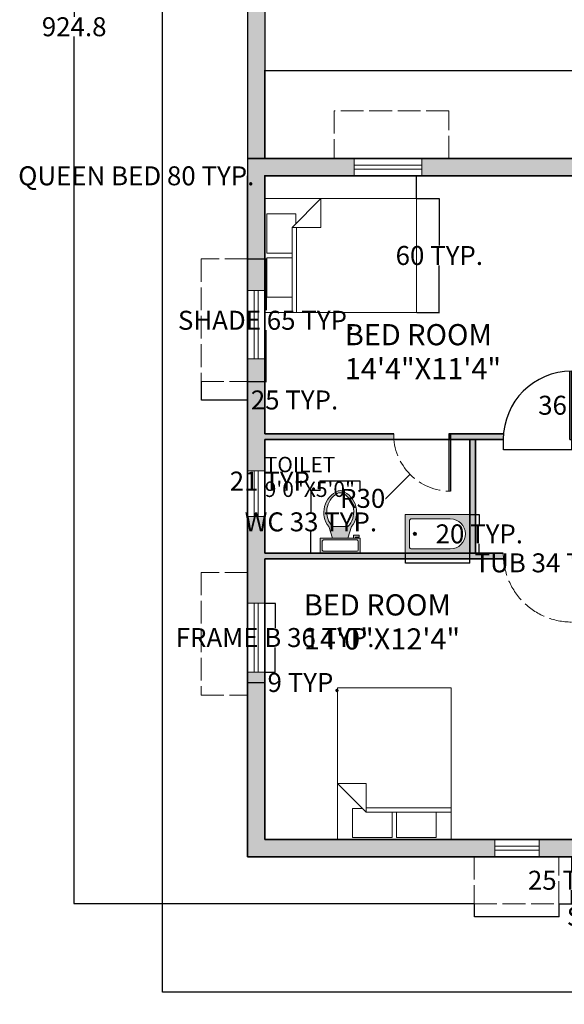
# Model space of a CAD drawing. Units: inches. Extents: x 215 to 969, y -612 to 418.
# Tile 1 of 8: x 215 to 502, y -612 to -93. Entities that reach past the tile are written whole.
import ezdxf

# ---------------------------------------------------------------- set-up
doc = ezdxf.new("R2010")
doc.units = ezdxf.units.IN
doc.header["$MEASUREMENT"] = 0
doc.linetypes.add('ACAD_ISO02W100', pattern=[15, 12, -3])
for name, color, linetype, lineweight in [('A-ANNO-DIMS', 2, 'Continuous', 18), ('A-AREA-IDEN', 7, 'Continuous', 18), ('A-DOOR', 3, 'Continuous', 25), ('A-DOOR-SWNG', 3, 'ACAD_ISO02W100', 13), ('A-FLOR-FIXT', 9, 'Continuous', 18), ('A-FLOR-OVHD', 8, 'ACAD_ISO02W100', 13), ('A-FLOR-SLAB', 7, 'Continuous', 25), ('A-FURN', 8, 'Continuous', 18), ('A-GLAZ', 4, 'Continuous', 18), ('A-WALL', 7, 'Continuous', 35)]:
    doc.layers.add(name, color=color, linetype=linetype, lineweight=lineweight)
doc.layers.add('A-WALL-PATT', color=252, linetype='Continuous', lineweight=13, true_color=0x939598)
doc.styles.get("Standard").update_dxf_attribs({"font": 'arial.ttf'})
doc.dimstyles.get("Standard").update_dxf_attribs({"dimtxt": 10, "dimasz": 0.18, "dimexe": 0.18, "dimexo": 0.0625, "dimgap": 0.09, "dimtad": 0, "dimtih": 1, "dimtoh": 1, "dimdec": 0, "dimzin": 0, "dimdsep": 46, "dimlunit": 3, "dimtxsty": 'Standard', "dimcen": 0.09, "dimadec": 0, "dimazin": 0, "dimtfac": 1, "dimtdec": 0, "dimtofl": 0, "dimtmove": 0, "dimatfit": 3, "dimfxl": 1, "dimtolj": 1, "dimtzin": 0, "dimarcsym": 0})

# ---------------------------------------------------------------- blocks, each defined once
blk = doc.blocks.new('Bed - Queen')
for p, q in [((0, -80.00003), (0, 0)), ((0, 0), (59.99999, 0)), ((59.99999, 0), (59.99999, -80.00003)), ((7.99999, -1.2), (28.79998, -1.2)), ((7.99999, -14.4), (7.99999, -1.2)), ((28.79998, -1.2), (28.79998, -14.4)), ((31.19999, -1.2), (51.99999, -1.2)), ((31.19999, -14.4), (31.19999, -1.2)), ((51.99999, -1.2), (51.99999, -16.4)), ((0, -14.4), (44.8, -14.4)), ((59.99999, -29.6), (44.8, -14.4)), ((44.8, -14.4), (44.8, -29.6)), ((44.8, -16.8), (0, -16.8)), ((51.99999, -16.4), (46.79936, -16.4)), ((44.8, -29.6), (59.99999, -29.6)), ((59.99999, -80.00003), (0, -80.00003))]:
    blk.add_line(p, q)
blk = doc.blocks.new('Bath Tub - 26 x 60 in.')
for p, q in [((8, -18), (10, -18)), ((9, -17), (9, -19))]:
    blk.add_line(p, q)
blk.add_lwpolyline([(0, -36), (0, 0), (60, 0), (60, -36)], close=True)
for points in [[(4, -30), (4, -6)], [(6, -4), (42, -4)], [(42, -32), (6, -32)]]:
    blk.add_lwpolyline(points)
for radius in [1.5, 1]:
    blk.add_circle((9, -18), radius)
for centre, radius, start, end in [((5.75, -5.75), 1.77, 81.8699, 188.1301), ((42, -18), 14, 270, 90), ((5.75, -30.25), 1.77, 171.8699, 278.1301)]:
    blk.add_arc(centre, radius, start, end)
blk = doc.blocks.new('Toilet - top')
for p, q in [((9.5, -6), (9.5, -2)), ((-10, -8.5), (-8, -8.5)), ((-10, -9.5), (-10, -8.5)), ((-7, -9.5), (-10, -9.5)), ((-8, -8.5), (-8, -8)), ((-7, -8), (-7, -9.5)), ((-4, -8), (-6, -14)), ((4, -8), (6, -14)), ((4, -14), (-4, -14))]:
    blk.add_line(p, q)
blk.add_lwpolyline([(10.5, -8), (10.5, 0), (-10.5, 0), (-10.5, -8)], close=True)
for points in [[(-9.5, -2), (-9.5, -6)], [(8.5, -1), (-8.5, -1)], [(-8.5, -7), (8.5, -7)]]:
    blk.add_lwpolyline(points)
for centre, radius, start, end in [((-8.62, -1.88), 0.884, 81.8699, 188.1301), ((8.62, -1.88), 0.884, 351.8699, 98.1301), ((-8.62, -6.12), 0.884, 171.8699, 278.1301), ((8.62, -6.12), 0.884, 261.8699, 8.1301), ((3.52, -21.58), 12.17, 141.4691, 247.9714), ((4.2, -21.82), 11.33, 136.3677, 238.9468), ((-3.52, -21.58), 12.17, 292.0284, 38.5307), ((-4.2, -21.82), 11.33, 301.053, 43.6321), ((0, -27.88), 4, 245.7318, 294.2682), ((0, -29), 4, 254.8605, 285.1395)]:
    blk.add_arc(centre, radius, start, end)
blk = doc.blocks.new('WINDOW-SHADE-60')
for p, q in [((60.48, 25.28), (0, 25.28)), ((0, 25.28), (0, 0)), ((60.48, 0), (60.48, 25.28))]:
    blk.add_line(p, q)
blk = doc.blocks.new('WINDOW-SHADE-65')
for p, q in [((24.53, 64.64), (0, 64.64)), ((0, 64.64), (0, 0)), ((0, 0), (24.53, 0))]:
    blk.add_line(p, q)
blk = doc.blocks.new('WINDOW-SHADE-45')
for p, q in [((0, 24.86), (0, 0)), ((44.63, 0), (44.63, 24.86)), ((0, 0), (44.63, 0))]:
    blk.add_line(p, q)
blk = doc.blocks.new('DOOR-SINGLE-36')
for p, q in [((35, 0), (35, 36)), ((36, 0), (36, 36)), ((35, 0), (36, 0))]:
    blk.add_line(p, q)
blk.add_arc((36, 0), 36, 90, 180)
blk = doc.blocks.new('WIN-24')
for p, q in [((0, 9), (0, 0)), ((0, 5.5), (23.37, 5.5)), ((23.37, 9), (23.37, 0)), ((0, 3.5), (23.37, 3.5))]:
    blk.add_line(p, q)
blk = doc.blocks.new('WIN-FRAME-24B')
for p, q in [((0, 23.99), (9, 23.99)), ((3.5, 23.99), (3.5, 0)), ((5.5, 23.99), (5.5, 0)), ((9, 0), (0, 0)), ((4.5, 0), (9, 0))]:
    blk.add_line(p, q)
blk = doc.blocks.new('WIN-FRAME-36A')
for p, q in [((0, 35.94), (9, 35.94)), ((3.5, 35.94), (3.5, 0)), ((5.5, 35.94), (5.5, 0)), ((9, 0), (0, 0)), ((4.5, 0), (9, 0))]:
    blk.add_line(p, q)
blk = doc.blocks.new('WIN-FRAME-36B')
for p, q in [((9, 36.42), (0, 36.42)), ((3.5, 36.42), (3.5, 0)), ((5.5, 36.42), (5.5, 0)), ((4.5, 0), (0, 0)), ((0, 0), (9, 0))]:
    blk.add_line(p, q)
blk = doc.blocks.new('*D23')
at = {"layer": 'A-ANNO-DIMS', "color": 0, "lineweight": -2, "transparency": 16777216}
for p, q in [((344.35, -175.5), (344.17, -175.5)), ((344.35, -187.44), (344.35, -175.32)), ((424.17, -175.5), (344.53, -175.5)), ((424.35, -187.44), (424.35, -175.32))]:
    blk.add_line(p, q, dxfattribs=at)
at = {"layer": 'A-ANNO-DIMS', "color": 0, "transparency": 16777216}
for points in [[(344.53, -175.47), (344.53, -175.53), (344.35, -175.5)], [(424.17, -175.47), (424.17, -175.53), (424.35, -175.5)]]:
    blk.add_solid(points, dxfattribs=at)
at = {"layer": 'Defpoints', "color": 0, "transparency": 16777216}
for p in [(344.35, -175.5), (344.35, -187.5), (424.35, -187.5)]:
    blk.add_point(p, dxfattribs=at)
at = {"layer": 'A-ANNO-DIMS', "color": 0, "transparency": 16777216, "insert": (276.67, -175.5), "char_height": 10, "attachment_point": 5}
blk.add_mtext('\\A1;QUEEN BED 80 TYP.', dxfattribs=at)
blk = doc.blocks.new('*D24')
at = {"layer": 'A-ANNO-DIMS', "color": 0, "lineweight": -2, "transparency": 16777216}
for p, q in [((424.42, -187.5), (436.53, -187.5)), ((436.35, -187.68), (436.35, -212.31)), ((436.35, -247.32), (436.35, -222.7)), ((424.42, -247.5), (436.53, -247.5))]:
    blk.add_line(p, q, dxfattribs=at)
at = {"layer": 'A-ANNO-DIMS', "color": 0, "transparency": 16777216}
for points in [[(436.32, -187.68), (436.38, -187.68), (436.35, -187.5)], [(436.32, -247.32), (436.38, -247.32), (436.35, -247.5)]]:
    blk.add_solid(points, dxfattribs=at)
at = {"layer": 'Defpoints', "color": 0, "transparency": 16777216}
for p in [(424.35, -187.5), (436.35, -187.5), (424.35, -247.5)]:
    blk.add_point(p, dxfattribs=at)
at = {"layer": 'A-ANNO-DIMS', "color": 0, "transparency": 16777216, "insert": (436.35, -217.5), "char_height": 10, "attachment_point": 5}
blk.add_mtext('\\A1;60 TYP.', dxfattribs=at)
blk = doc.blocks.new('*D25')
at = {"layer": 'A-ANNO-DIMS', "color": 0, "lineweight": -2, "transparency": 16777216}
for p, q in [((373.57, -341.41), (368.5, -341.41)), ((368.68, -341.59), (368.68, -352.67)), ((368.68, -374.27), (368.68, -363.19)), ((373.57, -374.45), (368.5, -374.45))]:
    blk.add_line(p, q, dxfattribs=at)
at = {"layer": 'A-ANNO-DIMS', "color": 0, "transparency": 16777216}
for points in [[(368.65, -341.59), (368.71, -341.59), (368.68, -341.41)], [(368.65, -374.27), (368.71, -374.27), (368.68, -374.45)]]:
    blk.add_solid(points, dxfattribs=at)
at = {"layer": 'Defpoints', "color": 0, "transparency": 16777216}
for p in [(373.64, -341.41), (368.68, -374.45), (373.64, -374.45)]:
    blk.add_point(p, dxfattribs=at)
at = {"layer": 'A-ANNO-DIMS', "color": 0, "transparency": 16777216, "insert": (368.68, -357.93), "char_height": 10, "attachment_point": 5}
blk.add_mtext('\\A1;WC 33 TYP.', dxfattribs=at)
blk = doc.blocks.new('*D26')
at = {"layer": 'A-ANNO-DIMS', "color": 0, "lineweight": -2, "transparency": 16777216}
for p, q in [((373.64, -336.45), (373.46, -336.45)), ((373.64, -341.34), (373.64, -336.27)), ((394.46, -336.45), (373.82, -336.45)), ((394.64, -341.34), (394.64, -336.27))]:
    blk.add_line(p, q, dxfattribs=at)
at = {"layer": 'A-ANNO-DIMS', "color": 0, "transparency": 16777216}
for points in [[(373.82, -336.42), (373.82, -336.48), (373.64, -336.45)], [(394.46, -336.42), (394.46, -336.48), (394.64, -336.45)]]:
    blk.add_solid(points, dxfattribs=at)
at = {"layer": 'Defpoints', "color": 0, "transparency": 16777216}
for p in [(373.64, -336.45), (373.64, -341.41), (394.64, -341.41)]:
    blk.add_point(p, dxfattribs=at)
at = {"layer": 'A-ANNO-DIMS', "color": 0, "transparency": 16777216, "insert": (348.94, -336.45), "char_height": 10, "attachment_point": 5}
blk.add_mtext('\\A1;21 TYP.', dxfattribs=at)
blk = doc.blocks.new('*D33')
at = {"layer": 'A-ANNO-DIMS', "color": 0, "lineweight": -2, "transparency": 16777216}
for p, q in [((418.41, -374.51), (418.41, -379.72)), ((452.34, -374.51), (452.34, -379.72)), ((418.59, -379.54), (452.16, -379.54)), ((452.34, -379.54), (452.52, -379.54))]:
    blk.add_line(p, q, dxfattribs=at)
at = {"layer": 'A-ANNO-DIMS', "color": 0, "transparency": 16777216}
for points in [[(418.59, -379.51), (418.59, -379.57), (418.41, -379.54)], [(452.16, -379.51), (452.16, -379.57), (452.34, -379.54)]]:
    blk.add_solid(points, dxfattribs=at)
at = {"layer": 'Defpoints', "color": 0, "transparency": 16777216}
for p in [(418.41, -374.45), (452.34, -374.45), (452.34, -379.54)]:
    blk.add_point(p, dxfattribs=at)
at = {"layer": 'A-ANNO-DIMS', "color": 0, "transparency": 16777216, "insert": (492.98, -379.54), "char_height": 10, "attachment_point": 5}
blk.add_mtext('\\A1;TUB 34 TYP.', dxfattribs=at)
blk = doc.blocks.new('*D34')
at = {"layer": 'A-ANNO-DIMS', "color": 0, "lineweight": -2, "transparency": 16777216}
for p, q in [((452.4, -354.09), (457.61, -354.09)), ((457.43, -354.27), (457.43, -359.08)), ((457.43, -374.27), (457.43, -369.47)), ((452.4, -374.45), (457.61, -374.45))]:
    blk.add_line(p, q, dxfattribs=at)
at = {"layer": 'A-ANNO-DIMS', "color": 0, "transparency": 16777216}
for points in [[(457.4, -354.27), (457.46, -354.27), (457.43, -354.09)], [(457.4, -374.27), (457.46, -374.27), (457.43, -374.45)]]:
    blk.add_solid(points, dxfattribs=at)
at = {"layer": 'Defpoints', "color": 0, "transparency": 16777216}
for p in [(452.34, -354.09), (457.43, -354.09), (452.34, -374.45)]:
    blk.add_point(p, dxfattribs=at)
at = {"layer": 'A-ANNO-DIMS', "color": 0, "transparency": 16777216, "insert": (457.43, -364.27), "char_height": 10, "attachment_point": 5}
blk.add_mtext('\\A1;20 TYP.', dxfattribs=at)
blk = doc.blocks.new('*D39')
at = {"layer": 'A-ANNO-DIMS', "color": 0, "lineweight": -2, "transparency": 16777216}
for p, q in [((470.07, -314.51), (470.07, -320.03)), ((506.07, -314.51), (506.07, -320.03)), ((470.25, -319.85), (505.89, -319.85)), ((506.07, -319.85), (506.25, -319.85))]:
    blk.add_line(p, q, dxfattribs=at)
at = {"layer": 'A-ANNO-DIMS', "color": 0, "transparency": 16777216}
for points in [[(470.25, -319.82), (470.25, -319.88), (470.07, -319.85)], [(505.89, -319.82), (505.89, -319.88), (506.07, -319.85)]]:
    blk.add_solid(points, dxfattribs=at)
at = {"layer": 'Defpoints', "color": 0, "transparency": 16777216}
for p in [(470.07, -314.45), (506.07, -314.45), (506.07, -319.85)]:
    blk.add_point(p, dxfattribs=at)
at = {"layer": 'A-ANNO-DIMS', "color": 0, "transparency": 16777216, "insert": (588.53, -319.85), "char_height": 10, "attachment_point": 5}
blk.add_mtext('\\A1;INTERIOR DOOR 36 TYP.', dxfattribs=at)
blk = doc.blocks.new('*D40')
at = {"layer": 'A-ANNO-DIMS', "color": 0, "lineweight": -2, "transparency": 16777216}
for p, q in [((506.13, -278.45), (511.65, -278.45)), ((511.47, -278.63), (511.47, -291.25)), ((511.47, -314.27), (511.47, -301.65)), ((506.13, -314.45), (511.65, -314.45))]:
    blk.add_line(p, q, dxfattribs=at)
at = {"layer": 'A-ANNO-DIMS', "color": 0, "transparency": 16777216}
for points in [[(511.44, -278.63), (511.5, -278.63), (511.47, -278.45)], [(511.44, -314.27), (511.5, -314.27), (511.47, -314.45)]]:
    blk.add_solid(points, dxfattribs=at)
at = {"layer": 'Defpoints', "color": 0, "transparency": 16777216}
for p in [(506.07, -278.45), (511.47, -278.45), (506.07, -314.45)]:
    blk.add_point(p, dxfattribs=at)
at = {"layer": 'A-ANNO-DIMS', "color": 0, "transparency": 16777216, "insert": (511.47, -296.45), "char_height": 10, "attachment_point": 5}
blk.add_mtext('\\A1;36 TYP.', dxfattribs=at)
blk = doc.blocks.new('*D59')
at = {"layer": 'A-ANNO-DIMS', "color": 0, "lineweight": -2, "transparency": 16777216}
for p, q in [((335.42, -219.33), (345.23, -219.33)), ((345.05, -219.51), (345.05, -246.39)), ((345.05, -283.79), (345.05, -256.91)), ((335.42, -283.97), (345.23, -283.97))]:
    blk.add_line(p, q, dxfattribs=at)
at = {"layer": 'A-ANNO-DIMS', "color": 0, "transparency": 16777216}
for points in [[(345.02, -219.51), (345.08, -219.51), (345.05, -219.33)], [(345.02, -283.79), (345.08, -283.79), (345.05, -283.97)]]:
    blk.add_solid(points, dxfattribs=at)
at = {"layer": 'Defpoints', "color": 0, "transparency": 16777216}
for p in [(335.35, -219.33), (345.05, -219.33), (335.35, -283.97)]:
    blk.add_point(p, dxfattribs=at)
at = {"layer": 'A-ANNO-DIMS', "color": 0, "transparency": 16777216, "insert": (345.05, -251.65), "char_height": 10, "attachment_point": 5}
blk.add_mtext('\\A1;SHADE 65 TYP.', dxfattribs=at)
blk = doc.blocks.new('*D60')
at = {"layer": 'A-ANNO-DIMS', "color": 0, "lineweight": -2, "transparency": 16777216}
for p, q in [((310.83, -284.03), (310.83, -293.85)), ((335.35, -284.03), (335.35, -293.85)), ((311.01, -293.67), (335.17, -293.67)), ((335.35, -293.67), (335.53, -293.67))]:
    blk.add_line(p, q, dxfattribs=at)
at = {"layer": 'A-ANNO-DIMS', "color": 0, "transparency": 16777216}
for points in [[(311.01, -293.64), (311.01, -293.7), (310.83, -293.67)], [(335.17, -293.64), (335.17, -293.7), (335.35, -293.67)]]:
    blk.add_solid(points, dxfattribs=at)
at = {"layer": 'Defpoints', "color": 0, "transparency": 16777216}
for p in [(310.83, -283.97), (335.35, -283.97), (335.35, -293.67)]:
    blk.add_point(p, dxfattribs=at)
at = {"layer": 'A-ANNO-DIMS', "color": 0, "transparency": 16777216, "insert": (360.05, -293.67), "char_height": 10, "attachment_point": 5}
blk.add_mtext('\\A1;25 TYP.', dxfattribs=at)
blk = doc.blocks.new('*D61')
at = {"layer": 'A-ANNO-DIMS', "color": 0, "lineweight": -2, "transparency": 16777216}
for p, q in [((454.72, -559.38), (454.72, -566.19)), ((499.35, -559.38), (499.35, -566.19)), ((454.9, -566.01), (499.17, -566.01)), ((499.35, -566.01), (499.53, -566.01))]:
    blk.add_line(p, q, dxfattribs=at)
at = {"layer": 'A-ANNO-DIMS', "color": 0, "transparency": 16777216}
for points in [[(454.9, -565.98), (454.9, -566.04), (454.72, -566.01)], [(499.17, -565.98), (499.17, -566.04), (499.35, -566.01)]]:
    blk.add_solid(points, dxfattribs=at)
at = {"layer": 'Defpoints', "color": 0, "transparency": 16777216}
for p in [(454.72, -559.31), (499.35, -559.31), (499.35, -566.01)]:
    blk.add_point(p, dxfattribs=at)
at = {"layer": 'A-ANNO-DIMS', "color": 0, "transparency": 16777216, "insert": (549.94, -566.01), "char_height": 10, "attachment_point": 5}
blk.add_mtext('\\A1;SHADE 45 TYP.', dxfattribs=at)
blk = doc.blocks.new('*D62')
at = {"layer": 'A-ANNO-DIMS', "color": 0, "lineweight": -2, "transparency": 16777216}
for p, q in [((499.42, -534.45), (506.23, -534.45)), ((506.05, -534.63), (506.05, -541.69)), ((506.05, -559.13), (506.05, -552.08)), ((499.42, -559.31), (506.23, -559.31))]:
    blk.add_line(p, q, dxfattribs=at)
at = {"layer": 'A-ANNO-DIMS', "color": 0, "transparency": 16777216}
for points in [[(506.02, -534.63), (506.08, -534.63), (506.05, -534.45)], [(506.02, -559.13), (506.08, -559.13), (506.05, -559.31)]]:
    blk.add_solid(points, dxfattribs=at)
at = {"layer": 'Defpoints', "color": 0, "transparency": 16777216}
for p in [(499.35, -534.45), (506.05, -534.45), (499.35, -559.31)]:
    blk.add_point(p, dxfattribs=at)
at = {"layer": 'A-ANNO-DIMS', "color": 0, "transparency": 16777216, "insert": (506.05, -546.88), "char_height": 10, "attachment_point": 5}
blk.add_mtext('\\A1;25 TYP.', dxfattribs=at)
blk = doc.blocks.new('*D67')
at = {"layer": 'A-ANNO-DIMS', "color": 0, "lineweight": -2, "transparency": 16777216}
for p, q in [((344.42, -400.71), (350, -400.71)), ((349.82, -400.89), (349.82, -413.72)), ((349.82, -436.96), (349.82, -424.12)), ((344.42, -437.14), (350, -437.14))]:
    blk.add_line(p, q, dxfattribs=at)
at = {"layer": 'A-ANNO-DIMS', "color": 0, "transparency": 16777216}
for points in [[(349.79, -400.89), (349.85, -400.89), (349.82, -400.71)], [(349.79, -436.96), (349.85, -436.96), (349.82, -437.14)]]:
    blk.add_solid(points, dxfattribs=at)
at = {"layer": 'Defpoints', "color": 0, "transparency": 16777216}
for p in [(344.35, -400.71), (349.82, -400.71), (344.35, -437.14)]:
    blk.add_point(p, dxfattribs=at)
at = {"layer": 'A-ANNO-DIMS', "color": 0, "transparency": 16777216, "insert": (349.82, -418.92), "char_height": 10, "attachment_point": 5}
blk.add_mtext('\\A1;FRAME B 36 TYP.', dxfattribs=at)
blk = doc.blocks.new('*D68')
at = {"layer": 'A-ANNO-DIMS', "color": 0, "lineweight": -2, "transparency": 16777216}
for p, q in [((335.35, -437.2), (335.35, -442.78)), ((344.35, -437.2), (344.35, -442.78)), ((335.53, -442.6), (344.17, -442.6)), ((344.35, -442.6), (344.53, -442.6))]:
    blk.add_line(p, q, dxfattribs=at)
at = {"layer": 'A-ANNO-DIMS', "color": 0, "transparency": 16777216}
for points in [[(335.53, -442.57), (335.53, -442.63), (335.35, -442.6)], [(344.17, -442.57), (344.17, -442.63), (344.35, -442.6)]]:
    blk.add_solid(points, dxfattribs=at)
at = {"layer": 'Defpoints', "color": 0, "transparency": 16777216}
for p in [(335.35, -437.14), (344.35, -437.14), (344.35, -442.6)]:
    blk.add_point(p, dxfattribs=at)
at = {"layer": 'A-ANNO-DIMS', "color": 0, "transparency": 16777216, "insert": (365.08, -442.6), "char_height": 10, "attachment_point": 5}
blk.add_mtext('\\A1;9 TYP.', dxfattribs=at)
blk = doc.blocks.new('*D69')
at = {"layer": 'A-ANNO-DIMS', "color": 0, "lineweight": -2, "transparency": 16777216}
for p, q in [((344.35, -166.39), (344.35, -119.87)), ((344.53, -120.05), (596.22, -120.05)), ((870.17, -120.05), (618.49, -120.05)), ((870.35, -166.39), (870.35, -119.87))]:
    blk.add_line(p, q, dxfattribs=at)
at = {"layer": 'A-ANNO-DIMS', "color": 0, "transparency": 16777216}
for points in [[(344.53, -120.02), (344.53, -120.08), (344.35, -120.05)], [(870.17, -120.02), (870.17, -120.08), (870.35, -120.05)]]:
    blk.add_solid(points, dxfattribs=at)
at = {"layer": 'Defpoints', "color": 0, "transparency": 16777216}
for p in [(870.35, -120.05), (344.35, -166.45), (870.35, -166.45)]:
    blk.add_point(p, dxfattribs=at)
at = {"layer": 'A-ANNO-DIMS', "color": 0, "transparency": 16777216, "insert": (607.35, -120.05), "char_height": 10, "attachment_point": 5}
blk.add_mtext('\\A1;526', dxfattribs=at)
blk = doc.blocks.new('*D75')
at = {"layer": 'A-ANNO-DIMS', "color": 0, "lineweight": -2, "transparency": 16777216}
for p, q in [((290.35, 103.15), (290.35, -605.89)), ((879.35, -534.51), (879.35, -605.89)), ((290.53, -605.71), (573.71, -605.71)), ((879.17, -605.71), (596, -605.71))]:
    blk.add_line(p, q, dxfattribs=at)
at = {"layer": 'A-ANNO-DIMS', "color": 0, "transparency": 16777216}
for points in [[(290.53, -605.68), (290.53, -605.74), (290.35, -605.71)], [(879.17, -605.68), (879.17, -605.74), (879.35, -605.71)]]:
    blk.add_solid(points, dxfattribs=at)
at = {"layer": 'Defpoints', "color": 0, "transparency": 16777216}
for p in [(290.35, 103.21), (879.35, -534.45), (879.35, -605.71)]:
    blk.add_point(p, dxfattribs=at)
at = {"layer": 'A-ANNO-DIMS', "color": 0, "transparency": 16777216, "insert": (584.85, -605.71), "char_height": 10, "attachment_point": 5}
blk.add_mtext('\\A1;589', dxfattribs=at)
blk = doc.blocks.new('*D76')
at = {"layer": 'A-ANNO-DIMS', "color": 0, "lineweight": -2, "transparency": 16777216}
for p, q in [((569.29, 365.5), (243.77, 365.5)), ((243.95, 365.32), (243.95, -91.71)), ((243.95, -559.13), (243.95, -102.1)), ((454.66, -559.31), (243.77, -559.31))]:
    blk.add_line(p, q, dxfattribs=at)
at = {"layer": 'A-ANNO-DIMS', "color": 0, "transparency": 16777216}
for points in [[(243.92, 365.32), (243.98, 365.32), (243.95, 365.5)], [(243.92, -559.13), (243.98, -559.13), (243.95, -559.31)]]:
    blk.add_solid(points, dxfattribs=at)
at = {"layer": 'Defpoints', "color": 0, "transparency": 16777216}
for p in [(569.35, 365.5), (243.95, -559.31), (454.72, -559.31)]:
    blk.add_point(p, dxfattribs=at)
at = {"layer": 'A-ANNO-DIMS', "color": 0, "transparency": 16777216, "insert": (243.95, -96.91), "char_height": 10, "attachment_point": 5}
blk.add_mtext('\\A1;924.8', dxfattribs=at)
blk = doc.blocks.new('*D86')
at = {"layer": 'A-ANNO-DIMS', "color": 0, "lineweight": -2, "transparency": 16777216}
for p, q in [((442.22, -311.81), (442.4, -311.81)), ((442.31, -311.9), (442.31, -311.72)), ((408.16, -345.55), (420.84, -333.02)), ((407.98, -345.55), (408.16, -345.55))]:
    blk.add_line(p, q, dxfattribs=at)
at = {"layer": 'A-ANNO-DIMS', "color": 0, "transparency": 16777216}
blk.add_solid([(420.82, -333), (420.86, -333.05), (420.97, -332.9)], dxfattribs=at)
at = {"layer": 'Defpoints', "color": 0, "transparency": 16777216}
for p in [(442.31, -311.81), (420.97, -332.9)]:
    blk.add_point(p, dxfattribs=at)
at = {"layer": 'A-ANNO-DIMS', "color": 0, "transparency": 16777216, "insert": (395.96, -345.55), "char_height": 10, "attachment_point": 5}
blk.add_mtext('\\A1;R30', dxfattribs=at)

msp = doc.modelspace()

# ---------------------------------------------------------------- hatches: boundary and pattern name
at = {"layer": 'A-WALL-PATT'}
h = msp.add_hatch(color=256, dxfattribs=at)
h.dxf.hatch_style = 1
h.paths.add_polyline_path([(764.0736, 322.2135), (569.3535, 322.2135), (565.0643, 322.2135), (565.0643, 313.2135), (569.3535, 313.2135), (569.3535, 205.2135), (509.3535, 205.2135), (509.3535, 247.2592), (506.3535, 247.2592), (506.3535, 172.2135), (491.3535, 172.2135), (491.3535, 169.2135), (509.3535, 169.2135), (509.3535, 202.2135), (569.3535, 202.2135), (569.3535, 169.2135), (578.3535, 169.2135), (578.3535, 205.2135), (578.3535, 237.2135), (615.7789, 237.2135), (615.7789, 246.2135), (578.3535, 246.2135), (578.3535, 313.2135), (710.3535, 313.2135), (710.3535, 246.2135), (710.3535, 211.3874), (719.3535, 211.3874), (719.3535, 295.2135), (719.3535, 313.2135), (764.0736, 313.2135)])
h.paths.add_polyline_path([(879.3535, 322.2135), (811.6486, 322.2135), (811.6486, 313.2135), (870.3535, 313.2135), (870.3535, 215.3905, -0.06325422), (879.3535, 216.5337), (879.3535, 313.2135)])
h.paths.add_polyline_path([(879.3535, 157.2135), (879.3535, 180.5337), (870.3535, 180.5337), (870.3535, 157.2135), (719.3535, 157.2135), (710.3535, 157.2135), (710.3535, 148.2135), (719.3535, 148.2135), (870.3535, 148.2135), (870.3535, 16.2135), (838.4933, 16.2135), (838.4933, 13.2135), (870.3535, 13.2135), (870.3535, -37.7865), (844.0345, -37.7865), (844.0345, -46.7865), (870.3535, -46.7865), (879.3535, -46.7865), (879.3535, -37.7865), (879.3535, 137.613)])
h.paths.add_polyline_path([(710.3535, 246.2135), (663.4146, 246.2135), (663.4146, 237.2135), (710.3535, 237.2135)], flags=17)
h.paths.add_polyline_path([(541.2942, 322.2135), (509.3535, 322.2135), (468.3222, 322.2135), (468.3222, 313.2135), (500.3535, 313.2135), (509.3535, 313.2135), (541.2942, 313.2135)])
h.paths.add_polyline_path([(509.3535, 313.2135), (503.3535, 313.2135), (503.3535, 277.5241, -0.04952579), (509.3535, 277.4203)], flags=17)
h.paths.add_polyline_path([(420.2828, 322.2135), (335.3535, 322.2135), (335.3535, 235.2487), (344.3535, 235.2487), (344.3535, 284.1885), (344.3535, 313.2135), (420.2828, 313.2135)])
h.paths.add_polyline_path([(335.3535, 181.2135), (290.3535, 181.2135), (290.3535, 103.2135), (335.3535, 103.2135), (335.3535, 112.2135), (299.3535, 112.2135), (299.3535, 129.1615), (299.3535, 172.2135), (335.3535, 172.2135)])
h.paths.add_polyline_path([(344.3535, 199.3097), (335.3535, 199.3097), (335.3535, 172.2135), (335.3535, 157.3369), (344.3535, 157.3369), (344.3535, 169.2135), (452.3535, 169.2135), (452.5037, 169.2135), (452.5037, 150.1199), (452.3535, 109.2135), (455.3535, 109.2135), (455.3535, 169.2135, -0.02086055), (455.4787, 172.2135), (344.3535, 172.2135)])
h.paths.add_polyline_path([(344.3535, 133.3441), (335.3535, 133.3441), (335.3535, 77.89), (344.3535, 77.89), (344.3535, 103.2135), (401.3556, 103.2135), (401.3556, 109.2135), (344.3535, 109.2135)])
h.paths.add_polyline_path([(462.6362, 109.2135), (443.0437, 109.2135), (425.2018, 109.2135), (425.2018, 106.2135), (452.3535, 106.2135), (462.7615, 106.2135, -0.02086055)])
h.paths.add_polyline_path([(540.3535, 106.2135), (684.3535, 106.2135), (684.3535, 35.7135), (687.3535, 35.7135), (687.3535, 56.1856), (693.3535, 56.1856), (693.3535, 109.2135), (540.3535, 109.2135), (531.3535, 109.2135), (498.6362, 109.2135), (498.6362, 106.2135), (531.3535, 106.2135), (531.3535, -37.7865), (507.9524, -37.7865), (507.9524, -46.7865), (610.6038, -46.7865), (610.6038, -37.7865), (540.3535, -37.7865)])
h.paths.add_polyline_path([(578.3535, 358.6622), (555.879, 358.6622), (555.879, 349.6622), (569.3535, 349.6622), (569.3535, 322.2135), (578.3535, 322.2135)])
h.paths.add_polyline_path([(525.962, 358.6622), (503.3535, 358.6622), (503.3535, 322.2135), (509.3535, 322.2135), (509.3535, 349.6622), (525.962, 349.6622)])
h.paths.add_polyline_path([(344.3535, 30.022), (335.3535, 30.022), (335.3535, -37.7865), (335.3535, -46.7865), (484.3302, -46.7865), (484.3302, -37.7865), (344.3535, -37.7865)])
h.paths.add_polyline_path([(719.1188, -37.7865), (698.4193, -37.7865), (693.3535, -37.7865), (693.3535, 7.424, -0.07717369), (684.3535, 6.0404), (684.3535, -37.7865), (658.8269, -37.7865), (658.8269, -46.7865), (684.3535, -46.7865), (684.3535, -82.7865), (693.3535, -82.7865), (704.1236, -82.7865), (704.1236, -78.0462), (693.3535, -78.0462), (693.3535, -46.7865), (719.1188, -46.7865)])
h.paths.add_polyline_path([(684.3535, -14.2202), (669.6716, -14.2202), (669.6716, -16.6044, -0.23606798), (667.6716, -17.6044), (667.6716, -18.6044, -0.11764706), (650.6716, -18.6044), (650.6716, -17.6044, -0.23606798), (648.6716, -16.6044), (648.6716, -14.2202), (603.0565, -14.2202), (603.0565, -37.7865), (684.3535, -37.7865)], flags=17)
h.paths.add_polyline_path([(665.6716, -14.2202), (652.6716, -14.2202), (652.6716, -16.6044, -0.23606798), (650.6716, -17.6044), (650.6716, -18.6044, 0.11764706), (667.6716, -18.6044), (667.6716, -17.6044, -0.23606798), (665.6716, -16.6044)], flags=16)
h.paths.add_polyline_path([(786.7385, -37.7865), (755.3535, -37.7865), (755.3535, 13.2135), (769.0808, 13.2135), (769.0808, 16.2135), (755.3535, 16.2135), (755.3535, 73.2135), (753.3535, 73.2135), (693.3535, 73.2135), (693.3535, 70.2135), (753.3535, 70.2135), (753.3535, -37.7865), (743.3062, -37.7865), (743.3062, -46.7865), (781.7385, -46.7865), (781.7385, -82.7865), (786.7385, -82.7865), (786.7385, -82.3744), (786.7385, -46.7865)])
h.paths.add_polyline_path([(844.0345, -37.7865), (786.7385, -37.7865), (786.7385, -46.7865), (844.0345, -46.7865)], flags=17)
h.paths.add_polyline_path([(781.7385, -78.0462), (704.1236, -78.0462), (704.1236, -82.7865), (781.7385, -82.7865)], flags=17)
h.paths.add_polyline_path([(344.3535, -46.7865), (335.3535, -46.7865), (335.3535, -166.4525), (344.3535, -166.4525)])
h.paths.add_polyline_path([(382.6632, 103.2135), (344.3535, 103.2135), (344.3535, 77.89), (344.3535, 32.7135), (363.5083, 32.7135), (382.6632, 32.7135)])
h.paths.add_polyline_path([(879.3535, -46.7865), (870.3535, -46.7865), (870.3535, -166.4525), (879.3535, -166.4525)])
h.paths.add_polyline_path([(879.3535, -166.4525), (799.4745, -166.4525), (799.4745, -175.4525), (855.3535, -175.4525), (870.3535, -175.4525), (870.3535, -192.5449), (879.3535, -192.5449), (879.3535, -175.4525)])
h.paths.add_polyline_path([(763.1775, -166.4525), (655.7214, -166.4525), (655.7214, -175.4525), (763.1775, -175.4525)])
h.paths.add_polyline_path([(619.8538, -166.4525), (550.8369, -166.4525), (550.8369, -175.4525), (619.8538, -175.4525)])
h.paths.add_polyline_path([(527.1282, -166.4525), (427.0819, -166.4525), (427.0819, -175.4525), (527.1282, -175.4525)])
h.paths.add_polyline_path([(391.4021, -166.4525), (335.3535, -166.4525), (335.3535, -175.4525), (335.3535, -236.0109), (344.3535, -236.0109), (344.3535, -187.5037), (344.3535, -175.4525), (391.4021, -175.4525)])
h.paths.add_polyline_path([(344.3535, -271.9249), (335.3535, -271.9249), (335.3535, -331.0209), (344.3535, -331.0209), (344.3535, -314.4525), (412.4218, -314.4525, -0.02503209), (412.3073, -311.4525), (344.3535, -311.4525)])
h.paths.add_polyline_path([(470.1954, -311.4525), (442.3073, -311.4525), (442.3073, -314.4525), (470.0702, -314.4525, -0.02086055)])
h.paths.add_polyline_path([(455.3535, -314.4525), (452.3535, -314.4525), (452.3535, -374.4525), (455.3535, -374.4525)])
h.paths.add_polyline_path([(579.3535, -241.4072), (519.3535, -241.4072), (519.3535, -283.4525), (579.3535, -283.4525)])
h.paths.add_polyline_path([(516.5043, -281.1089), (584.3098, -281.1089), (584.3098, -264.0138), (516.5043, -264.0138)], flags=9)
h.paths.add_polyline_path([(516.4662, -263.2183), (581.1504, -263.2183), (581.1504, -245.8948), (516.4662, -245.8948)], flags=9)
h = msp.add_hatch(color=256, dxfattribs=at)
h.dxf.hatch_style = 1
h.paths.add_polyline_path([(723.3535, -175.4525), (714.3535, -175.4525), (714.3535, -205.9065), (720.3535, -205.9065), (720.3535, -314.4525), (723.3535, -314.4525)])
h.paths.add_polyline_path([(720.3535, -311.4525), (714.3535, -311.4525), (714.3535, -314.4525), (720.3535, -314.4525)], flags=17)
h.paths.add_polyline_path([(879.3535, -228.5449, -0.06325422), (870.3535, -227.4017), (870.3535, -314.4525), (870.3535, -410.4525), (870.3535, -464.8456), (870.3535, -525.4525), (730.3535, -525.4525), (730.3535, -473.8456), (753.1403, -473.8456), (753.1403, -464.8456), (686.9324, -464.8456), (686.9324, -473.8456), (721.3535, -473.8456), (721.3535, -525.4525), (594.3535, -525.4525), (594.3535, -473.8456), (622.1543, -473.8456), (622.1543, -464.8456), (594.3535, -464.8456), (594.3535, -414.4525), (525.3535, -414.4525), (525.3535, -417.4525), (585.3535, -417.4525), (585.3535, -525.4525), (571.9682, -525.4525), (571.9682, -534.4525), (879.3535, -534.4525), (879.3535, -410.4525), (879.3535, -314.4525)])
h.paths.add_polyline_path([(730.3535, -368.8456), (870.3535, -368.8456), (870.3535, -365.8456), (721.3535, -365.8456), (721.3535, -368.8456), (721.3535, -409.1143), (730.3535, -409.1143)], flags=17)
h.paths.add_polyline_path([(870.3535, -410.4525), (870.3535, -368.8456), (763.5487, -368.8456), (763.5487, -393.1792), (831.3894, -393.1792), (831.3894, -438.7284), (789.7386, -438.7284), (789.7386, -464.8456), (870.3535, -464.8456)], flags=17)
h.paths.add_polyline_path([(839.0857, -434.8848), (839.0857, -399.5193), (865.1757, -399.5193), (865.1757, -434.8848)], flags=16)
h.paths.add_polyline_path([(839.8092, -427.6923, -0.48074962), (841.3551, -426.456, -0.48074962), (842.901, -427.6923, -0.48074962), (841.3551, -428.9285, -0.48074962)], flags=0)
h.paths.add_polyline_path([(848.5001, -427.1588, -0.44021274), (854.7228, -421.4606, -0.49540019), (861.9637, -426.9752, -0.44021274), (855.741, -432.6734, -0.49540019)], flags=0)
h.paths.add_polyline_path([(848.5001, -410.0762, -0.44021274), (854.7228, -404.378, -0.49540019), (861.9637, -409.8925, -0.44021274), (855.741, -415.5907, -0.49540019)], flags=0)
h.paths.add_polyline_path([(839.8092, -410.149, -0.48074962), (841.3551, -408.9127, -0.48074962), (842.901, -410.149, -0.48074962), (841.3551, -411.3852, -0.48074962)], flags=0)
h.paths.add_polyline_path([(870.3535, -464.8456), (789.7386, -464.8456), (789.1403, -464.8456, -0.06325422), (787.9971, -473.8456), (870.3535, -473.8456)], flags=17)
h.paths.add_polyline_path([(727.9401, -444.9303), (724.3796, -444.9303), (724.3796, -464.8456), (727.9401, -464.8456)], flags=17)
h.paths.add_polyline_path([(548.597, -525.4525), (531.2503, -525.4525), (525.3535, -525.4525), (525.3535, -490.3641, -0.07632083), (516.3535, -491.7459), (516.3535, -525.4525), (488.9462, -525.4525), (488.9462, -534.4525), (548.597, -534.4525)])
h.paths.add_polyline_path([(525.3535, -374.4525), (506.0702, -374.4525), (506.0702, -377.4525), (516.3535, -377.4525), (516.3535, -461.7459), (519.3535, -461.7459), (519.3535, -417.4525), (525.3535, -417.4525), (525.3535, -414.4525)])
h.paths.add_polyline_path([(470.1724, -377.4525), (449.6899, -377.4525), (344.3535, -377.4525), (344.3535, -400.7118), (335.3535, -400.7118), (335.3535, -355.0472), (344.3535, -355.0472), (344.3535, -374.4525), (373.6368, -374.4525), (373.6368, -366.4525), (380.1368, -366.4525), (378.1369, -360.4526, -0.50132349), (383.0921, -341.5914, -0.13289091), (385.1815, -341.5914, -0.50131678), (390.1369, -360.4524), (388.1368, -366.4525), (391.1368, -366.4525), (391.1368, -364.9525), (394.1368, -364.9525), (394.1368, -365.9525), (392.1368, -365.9525), (392.1368, -366.4525), (394.6368, -366.4525), (394.6368, -374.4525), (418.4066, -374.4525), (418.4066, -354.0926), (452.3535, -354.0926), (452.3535, -374.4525), (470.0713, -374.4525, 0.02085422)])
h.paths.add_polyline_path([(442.1598, -372.1903), (421.7999, -372.1903, -0.50000012), (420.6688, -371.0592), (420.6688, -357.4859, -0.50000012), (421.7999, -356.3548), (442.1598, -356.3548, -1)], flags=16)
h.paths.add_polyline_path([(422.6483, -364.2725, -1), (424.3449, -364.2725, -1)], flags=0)
h.paths.add_polyline_path([(422.931, -364.2725, -1), (424.0621, -364.2725, -1)], flags=0)
h.paths.add_polyline_path([(392.6368, -373.4525), (375.6368, -373.4525, -0.50000012), (374.6368, -372.4525), (374.6368, -368.4525, -0.50000012), (375.6368, -367.4525), (392.6368, -367.4525, -0.50000012), (393.6368, -368.4525), (393.6368, -372.4525, -0.50000012)], flags=16)
h.paths.add_polyline_path([(388.1368, -360.4525), (380.1368, -360.4525, -0.4800795), (382.4928, -342.9295, -0.21500378), (385.7809, -342.9295, -0.48007965)], flags=16)
h.paths.add_polyline_path([(344.3535, -437.1356), (335.3535, -437.1356), (335.3535, -525.4525), (335.3535, -534.4525), (465.575, -534.4525), (465.575, -525.4525), (344.3535, -525.4525)])
h.paths.add_polyline_path([(342.2824, -347.0067), (391.5718, -347.0067), (391.5718, -334.5799), (342.2824, -334.5799)], flags=9)

# ---------------------------------------------------------------- linework, layer by layer
at = {"layer": 'A-DOOR'}
for p, q in [((442.3073, -311.4525), (441.3073, -311.4525)), ((441.3073, -311.4525), (441.3073, -341.8122)), ((442.3073, -314.4525), (442.3073, -311.4525)), ((442.3073, -311.4525), (442.3073, -341.8122))]:
    msp.add_line(p, q, dxfattribs=at)
at = {"layer": 'A-DOOR-SWNG'}
for centre, radius, start in [((442.3073, -311.8101), 30.0021, 179.317089), ((506.0702, -374.7412), 36, 179.540554)]:
    msp.add_arc(centre, radius, start, 270, dxfattribs=at)
at = {"layer": 'A-FLOR-SLAB'}
for p, q in [((335.3535, -46.7865), (335.3535, -175.4525)), ((344.3535, -46.7865), (344.3535, -166.4525))]:
    msp.add_line(p, q, dxfattribs=at)
at = {"layer": 'A-WALL'}
for p, q in [((335.3535, -166.4525), (879.3535, -166.4525)), ((335.3535, -175.4525), (335.3535, -311.4525)), ((344.3535, -175.4525), (870.3535, -175.4525)), ((344.3535, -175.4525), (344.3535, -311.4525)), ((335.3535, -525.4525), (335.3535, -271.9249)), ((335.3535, -314.4525), (335.3535, -374.4525)), ((344.3535, -311.4525), (412.3073, -311.4525)), ((344.3535, -314.4525), (470.0702, -314.4525)), ((344.3535, -314.4525), (344.3535, -374.4525)), ((441.3073, -311.4525), (470.1954, -311.4525)), ((452.3535, -374.4525), (452.3535, -314.4525)), ((455.3535, -374.4525), (455.3535, -314.4525)), ((335.3535, -377.4525), (335.3535, -525.4525)), ((344.3535, -374.4525), (452.3535, -374.4525)), ((344.3535, -377.4525), (452.3535, -377.4525)), ((344.3535, -377.4525), (344.3535, -525.4525)), ((470.0713, -374.4525), (449.6899, -374.4525)), ((470.1724, -377.4525), (449.6899, -377.4525)), ((335.3535, -534.4525), (335.3535, -525.4525)), ((344.3535, -525.4525), (516.3535, -525.4525)), ((879.3535, -534.4525), (335.3535, -534.4525)), ((344.3535, -534.4525), (516.3535, -534.4525))]:
    msp.add_line(p, q, dxfattribs=at)

# ---------------------------------------------------------------- block references
at = {"layer": 'A-DOOR'}
msp.add_blockref('DOOR-SINGLE-36', (470.0697, -314.452), dxfattribs=at)
at = {"layer": 'A-FLOR-FIXT', "rotation": 180}
msp.add_blockref('Toilet - top', (384.1368, -374.4525), dxfattribs=at)
at = {"layer": 'A-FLOR-FIXT', "xscale": 0.5655524882750257, "yscale": 0.5655524882750257, "zscale": 0.5655524882750257}
msp.add_blockref('Bath Tub - 26 x 60 in.', (418.4066, -354.0926), dxfattribs=at)
at = {"layer": 'A-FLOR-OVHD'}
for name, p in [('WINDOW-SHADE-60', (380.9601, -166.452)), ('WINDOW-SHADE-65', (310.827, -283.971)), ('WINDOW-SHADE-65', (310.827, -449.2252)), ('WINDOW-SHADE-45', (454.722, -559.313))]:
    msp.add_blockref(name, p, dxfattribs=at)
at = {"layer": 'A-FURN'}
for p, rotation in [((344.3535, -247.5037), 90), ((442.6437, -525.4525), 180)]:
    msp.add_blockref('Bed - Queen', p, dxfattribs=dict(at, rotation=rotation))
at = {"layer": 'A-GLAZ', "yscale": 0.9927843475025763, "rotation": 90}
msp.add_blockref('WIN-FRAME-36A', (427.0815, -175.453), dxfattribs=at)
at = {"layer": 'A-GLAZ', "extrusion": (0, 0, -1), "zscale": -1, "rotation": 180}
for name, p, yscale in [('WIN-FRAME-36A', (-335.353, -236.0113), 0.9993009930512943), ('WIN-FRAME-24B', (-335.353, -331.0208), 1.001396274826156)]:
    msp.add_blockref(name, p, dxfattribs=dict(at, yscale=yscale))
at = {"layer": 'A-GLAZ'}
for name, p in [('WIN-FRAME-36B', (335.353, -437.136)), ('WIN-24', (465.575, -534.452))]:
    msp.add_blockref(name, p, dxfattribs=at)

# ---------------------------------------------------------------- texts
at = {"layer": 'A-AREA-IDEN'}
for s, height, p in [('BED ROOM', 11.16071, (386.5819, -264.8324)), ('14\'4"X11\'4"', 11.160707, (386.5819, -282.7611)), ('TOILET', 8.11299, (344.3535, -331.7644)), ('9\'0"X5\'0"', 8.11299, (344.3535, -344.7972)), ('BED ROOM', 11.16071, (365.0052, -407.2906)), ('14\'0"X12\'4"', 11.160707, (365.0052, -425.2193))]:
    msp.add_text(s, height=height, dxfattribs=at).set_placement(p)

# ---------------------------------------------------------------- dimensions: what is measured, and where the dimension line sits
at = {"layer": 'A-ANNO-DIMS'}
dim = msp.add_linear_dim(base=(243.9535, -559.3132), p1=(569.3535, 365.5008), p2=(454.7218, -559.3132), angle=90, dimstyle='Standard', override={"dimdec": 1, "dimlfac": 1, "dimrnd": 0, "dimzin": 0, "dimdsep": 46, "dimlunit": 2}, dxfattribs=at)
dim.commit()
dim.dimension.update_dxf_attribs({"geometry": '*D76', "text_midpoint": (243.9535, -96.9062)})
for base, p1, p2, picture, middle in [((879.3535, -605.7132), (290.3535, 103.2135), (879.3535, -534.4525), '*D75', (584.8535, -605.7132)), ((870.3535, -120.0525), (344.3535, -166.4525), (870.3535, -166.4525), '*D69', (607.3535, -120.0525))]:
    dim = msp.add_linear_dim(base=base, p1=p1, p2=p2, dimstyle='Standard', override={"dimdec": 0, "dimlfac": 1, "dimrnd": 0, "dimzin": 0, "dimdsep": 46, "dimlunit": 2}, dxfattribs=at)
    dim.commit()
    dim.dimension.update_dxf_attribs({"geometry": picture, "text_midpoint": middle})
for base, p1, p2, angle, text, picture, middle in [((344.3535, -175.5037), (424.3535, -187.5037), (344.3535, -187.5037), 180, 'QUEEN BED <> TYP.', '*D23', (276.6722, -175.5037)), ((436.3535, -187.5037), (424.3535, -247.5037), (424.3535, -187.5037), 90, '<> TYP.', '*D24', (436.3535, -217.5037)), ((345.0493, -219.3322), (335.3535, -283.9708), (335.3535, -219.3322), 90, 'SHADE <> TYP.', '*D59', (345.0493, -251.6515)), ((511.4702, -278.4525), (506.0702, -314.4525), (506.0702, -278.4525), 90, '<> TYP.', '*D40', (511.4702, -296.4525)), ((373.6368, -336.4493), (394.6368, -341.4063), (373.6368, -341.4063), 180, '<> TYP.', '*D26', (348.9432, -336.4493)), ((368.6799, -374.4525), (373.6368, -341.4063), (373.6368, -374.4525), 270, 'WC <> TYP.', '*D25', (368.6799, -357.9294)), ((457.4297, -354.0926), (452.3398, -374.4525), (452.3398, -354.0926), 90, '<> TYP.', '*D34', (457.4297, -364.2725)), ((349.8171, -400.7118), (344.3535, -437.1356), (344.3535, -400.7118), 90, 'FRAME B <> TYP.', '*D67', (349.8171, -418.9237)), ((506.0478, -534.4525), (499.3531, -559.3132), (499.3531, -534.4525), 90, '<> TYP.', '*D62', (506.0478, -546.8828))]:
    dim = msp.add_linear_dim(base=base, p1=p1, p2=p2, angle=angle, text=text, dimstyle='Standard', override={"dimdec": 0, "dimlfac": 1, "dimrnd": 0, "dimzin": 0, "dimdsep": 46, "dimlunit": 2}, dxfattribs=at)
    dim.commit()
    dim.dimension.update_dxf_attribs({"geometry": picture, "text_midpoint": middle})
for base, p1, p2, text, picture, middle in [((335.3535, -293.6666), (310.8275, -283.9708), (335.3535, -283.9708), '<> TYP.', '*D60', (360.0471, -293.6666)), ((506.0702, -319.8525), (470.0702, -314.4525), (506.0702, -314.4525), 'INTERIOR DOOR <> TYP.', '*D39', (588.5264, -319.8525)), ((452.3398, -379.5425), (418.4066, -374.4525), (452.3398, -374.4525), 'TUB <> TYP.', '*D33', (492.9849, -379.5425)), ((344.3535, -442.5992), (335.3535, -437.1356), (344.3535, -437.1356), '<> TYP.', '*D68', (365.0771, -442.5992)), ((499.3531, -566.0078), (454.7218, -559.3132), (499.3531, -559.3132), 'SHADE <> TYP.', '*D61', (549.9437, -566.0078))]:
    dim = msp.add_linear_dim(base=base, p1=p1, p2=p2, text=text, dimstyle='Standard', override={"dimdec": 0, "dimlfac": 1, "dimrnd": 0, "dimzin": 0, "dimdsep": 46, "dimlunit": 2}, dxfattribs=at)
    dim.commit()
    dim.dimension.update_dxf_attribs({"geometry": picture, "text_midpoint": middle})
dim = msp.add_radius_dim(center=(442.3073, -311.8101), mpoint=(420.9668, -332.8982), dimstyle='Standard', override={"dimdec": 0, "dimlfac": 1, "dimrnd": 0, "dimzin": 0, "dimdsep": 46, "dimlunit": 2}, dxfattribs=at)
dim.commit()
dim.dimension.update_dxf_attribs({"geometry": '*D86', "text_midpoint": (395.962, -345.5511), "dimtype": 164})

doc.saveas('drawing.dxf')
